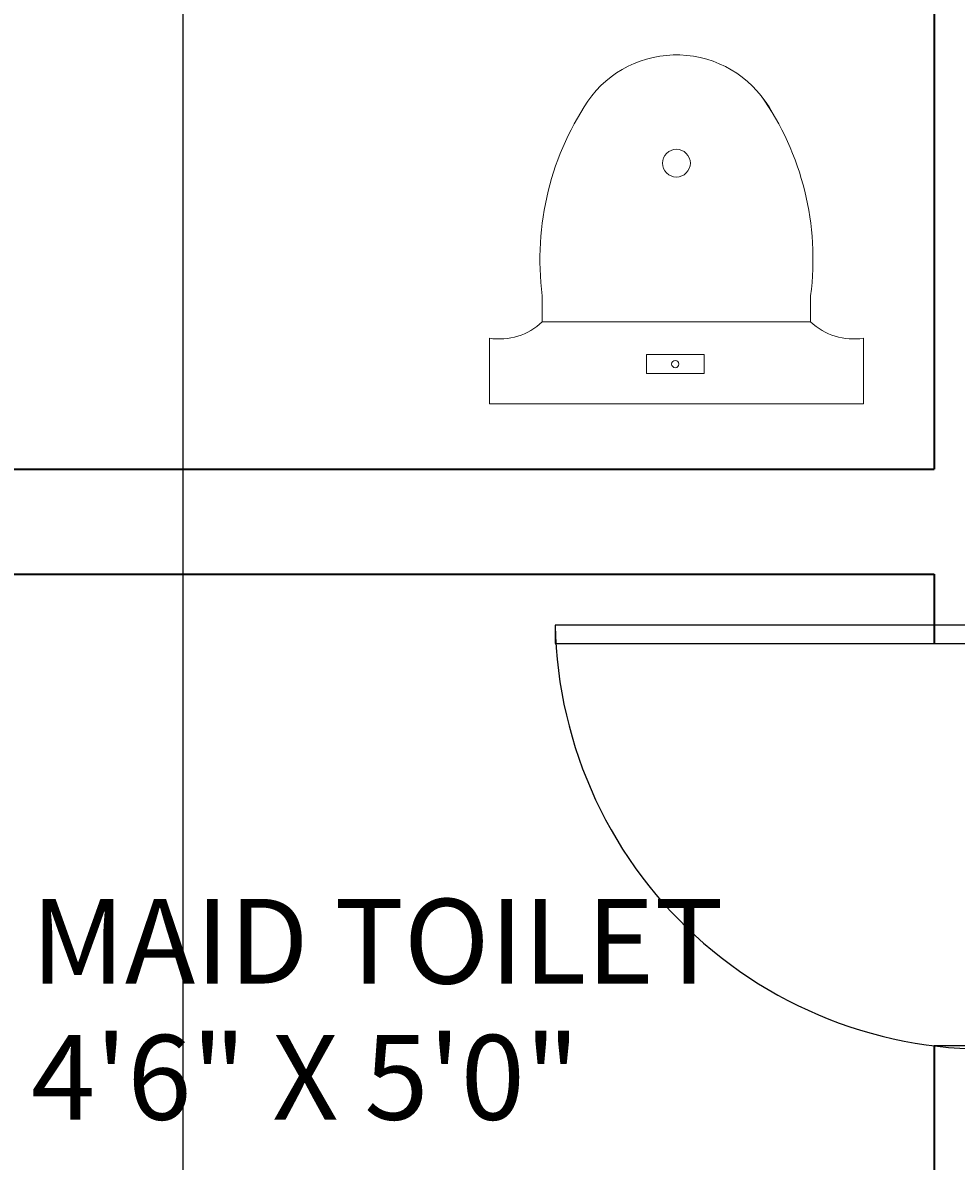
# Model space of a CAD drawing. Units: inches. Extents: x -61 to 1599, y -1316 to 257.
# Tile 84 of 204: x 268 to 321, y -407 to -342. Entities that reach past the tile are written whole.
import ezdxf

# ---------------------------------------------------------------- set-up
doc = ezdxf.new("R2010")
doc.units = ezdxf.units.IN
doc.header["$MEASUREMENT"] = 0
doc.linetypes.add('ACAD_ISO02W100', pattern=[15, 12, -3])
for name, color, linetype, lineweight in [('A-ANNO-DIMS', 2, 'Continuous', 18), ('A-AREA-IDEN', 1, 'Continuous', 18), ('A-FLOR-FIXT', 8, 'Continuous', 18), ('A-WALL-JAMB', 4, 'ACAD_ISO02W100', 25), ('DOORS', 2, 'Continuous', 25), ('WALLS', 4, 'Continuous', 35)]:
    doc.layers.add(name, color=color, linetype=linetype, lineweight=lineweight)
doc.styles.get("Standard").update_dxf_attribs({"font": 'arial.ttf'})
doc.dimstyles.get("Standard").update_dxf_attribs({"dimtxt": 0.18, "dimasz": 0.18, "dimexe": 0.18, "dimexo": 0.0625, "dimgap": 0.09, "dimtad": 0, "dimtih": 1, "dimtoh": 1, "dimdec": 0, "dimzin": 0, "dimdsep": 46, "dimlunit": 3, "dimtxsty": 'Standard', "dimcen": 0.09, "dimadec": 0, "dimazin": 0, "dimtfac": 1, "dimtdec": 0, "dimtofl": 0, "dimtmove": 0, "dimatfit": 3, "dimfxl": 1, "dimtolj": 1, "dimtzin": 0, "dimarcsym": 0})

# ---------------------------------------------------------------- blocks, each defined once
blk = doc.blocks.new('DOOR-SWING-24')
blk.add_line((0, 0), (0, 3.6))
blk.add_lwpolyline([(0, 0), (0, -24), (1.05, -24), (1.05, 0)], close=True)
blk.add_arc((-0.441, 0.618), 24.622, 271.02591, 6.95592)
blk = doc.blocks.new('WC-FLOOR-MOUNT')
for p, q in [((3.018, 4.686), (3.018, 6.173)), ((18.314, 4.686), (18.314, 6.173)), ((3.018, 4.686), (18.314, 4.686)), ((0, 0), (0, 3.747)), ((21.331, 0), (21.331, 3.747)), ((0, 0), (21.331, 0))]:
    blk.add_line(p, q)
blk.add_lwpolyline([(12.243, 1.734), (8.955, 1.734), (8.955, 2.812), (12.243, 2.812)], close=True)
for centre, radius in [((10.666, 13.729), 0.792), ((10.599, 2.273), 0.208)]:
    blk.add_circle(centre, radius)
for centre, radius, start, end in [((10.666, 13.729), 6.176, 27.68441, 141.46969), ((19.051, 8.262), 16.169, 144.82396, 187.42318), ((2.281, 8.262), 16.169, 352.57682, 35.17604), ((0.565, 7.253), 3.551, 260.8586, 313.6993), ((20.767, 7.253), 3.551, 226.3007, 279.1414)]:
    blk.add_arc(centre, radius, start, end)
blk = doc.blocks.new('*D687')
at = {"layer": 'A-ANNO-DIMS', "color": 0, "lineweight": -2, "transparency": 16777216}
for p, q in [((289.418, 181.677), (-61.077, 181.677)), ((-60.897, 181.497), (-60.897, -528.952)), ((-60.897, -1239.765), (-60.897, -529.316)), ((319.64, -1239.945), (-61.077, -1239.945))]:
    blk.add_line(p, q, dxfattribs=at)
at = {"layer": 'A-ANNO-DIMS', "color": 0, "transparency": 16777216}
for points in [[(-60.927, 181.497), (-60.867, 181.497), (-60.897, 181.677)], [(-60.927, -1239.765), (-60.867, -1239.765), (-60.897, -1239.945)]]:
    blk.add_solid(points, dxfattribs=at)
at = {"layer": 'DEFPOINTS', "color": 0, "transparency": 16777216}
for p in [(289.481, 181.677), (-60.897, -1239.945), (319.703, -1239.945)]:
    blk.add_point(p, dxfattribs=at)
at = {"layer": 'A-ANNO-DIMS', "color": 0, "transparency": 16777216, "insert": (-60.897, -529.134), "char_height": 0.18, "attachment_point": 5}
blk.add_mtext('\\A1;1421.6', dxfattribs=at)
blk = doc.blocks.new('*D699')
at = {"layer": 'A-ANNO-DIMS', "color": 0, "lineweight": -2, "transparency": 16777216}
for p, q in [((835.64, -167.169), (-61.077, -167.169)), ((-60.897, -167.349), (-60.897, -306.726)), ((-60.897, -446.466), (-60.897, -307.09)), ((841.64, -446.646), (-61.077, -446.646))]:
    blk.add_line(p, q, dxfattribs=at)
at = {"layer": 'A-ANNO-DIMS', "color": 0, "transparency": 16777216}
for points in [[(-60.927, -167.349), (-60.867, -167.349), (-60.897, -167.169)], [(-60.927, -446.466), (-60.867, -446.466), (-60.897, -446.646)]]:
    blk.add_solid(points, dxfattribs=at)
at = {"layer": 'DEFPOINTS', "color": 0, "transparency": 16777216}
for p in [(835.703, -167.169), (-60.897, -446.646), (841.703, -446.646)]:
    blk.add_point(p, dxfattribs=at)
at = {"layer": 'A-ANNO-DIMS', "color": 0, "transparency": 16777216, "insert": (-60.897, -306.908), "char_height": 0.18, "attachment_point": 5}
blk.add_mtext('\\A1;279.5', dxfattribs=at)
blk = doc.blocks.new('*D702')
at = {"layer": 'A-ANNO-DIMS', "color": 0, "lineweight": -2, "transparency": 16777216}
for p, q in [((276.882, -616.882), (276.882, 257.457)), ((277.062, 257.277), (312.209, 257.277)), ((348.14, 257.277), (312.994, 257.277)), ((348.32, -616.882), (348.32, 257.457))]:
    blk.add_line(p, q, dxfattribs=at)
at = {"layer": 'A-ANNO-DIMS', "color": 0, "transparency": 16777216}
for points in [[(277.062, 257.307), (277.062, 257.247), (276.882, 257.277)], [(348.14, 257.307), (348.14, 257.247), (348.32, 257.277)]]:
    blk.add_solid(points, dxfattribs=at)
at = {"layer": 'DEFPOINTS', "color": 0, "transparency": 16777216}
for p in [(348.32, 257.277), (276.882, -616.945), (348.32, -616.945)]:
    blk.add_point(p, dxfattribs=at)
at = {"layer": 'A-ANNO-DIMS', "color": 0, "transparency": 16777216, "insert": (312.601, 257.277), "char_height": 0.18, "attachment_point": 5}
blk.add_mtext('\\A1;71.44', dxfattribs=at)

msp = doc.modelspace()

# ---------------------------------------------------------------- linework, layer by layer
at = {"layer": 'A-WALL-JAMB'}
for p, q in [((325.7028, -376.2211), (319.7028, -376.2211)), ((325.7028, -400.2211), (319.7028, -400.2211))]:
    msp.add_line(p, q, dxfattribs=at)
at = {"layer": 'WALLS'}
for p, q in [((319.7028, -288.3229), (319.7028, -367.3229)), ((265.7028, -367.3229), (319.7028, -367.3229)), ((265.7028, -373.3229), (319.7028, -373.3229)), ((319.7028, -373.3229), (319.7028, -377.2711)), ((319.7028, -400.2167), (319.7028, -432.3229))]:
    msp.add_line(p, q, dxfattribs=at)

# ---------------------------------------------------------------- block references
at = {"layer": 'A-FLOR-FIXT'}
msp.add_blockref('WC-FLOOR-MOUNT', (294.349, -363.6106), dxfattribs=at)
at = {"layer": 'DOORS', "rotation": 270}
msp.add_blockref('DOOR-SWING-24', (322.1028, -376.2211), dxfattribs=at)

# ---------------------------------------------------------------- texts
at = {"layer": 'A-AREA-IDEN'}
for s, p in [('MAID TOILET', (268.2172, -396.6681)), ('4\'6" X 5\'0"', (268.2172, -404.4305))]:
    msp.add_text(s, height=4.832098, dxfattribs=at).set_placement(p)

# ---------------------------------------------------------------- dimensions: what is measured, and where the dimension line sits
at = {"layer": 'A-ANNO-DIMS'}
dim = msp.add_linear_dim(base=(348.3201, 257.2771), p1=(276.8825, -616.9446), p2=(348.3201, -616.9446), dimstyle='Standard', override={"dimdec": 2, "dimlfac": 1, "dimrnd": 0, "dimzin": 0, "dimdsep": 46, "dimlunit": 2}, dxfattribs=at)
dim.commit()
dim.dimension.update_dxf_attribs({"geometry": '*D702', "text_midpoint": (312.6013, 257.2771)})
for base, p1, p2, picture, middle in [((-60.8972, -1239.9446), (289.4807, 181.6771), (319.7028, -1239.9446), '*D687', (-60.8972, -529.1337)), ((-60.8972, -446.6462), (835.7028, -167.169), (841.7028, -446.6462), '*D699', (-60.8972, -306.9076))]:
    dim = msp.add_linear_dim(base=base, p1=p1, p2=p2, angle=90, dimstyle='Standard', override={"dimdec": 1, "dimlfac": 1, "dimrnd": 0, "dimzin": 0, "dimdsep": 46, "dimlunit": 2}, dxfattribs=at)
    dim.commit()
    dim.dimension.update_dxf_attribs({"geometry": picture, "text_midpoint": middle})

doc.saveas('drawing.dxf')
